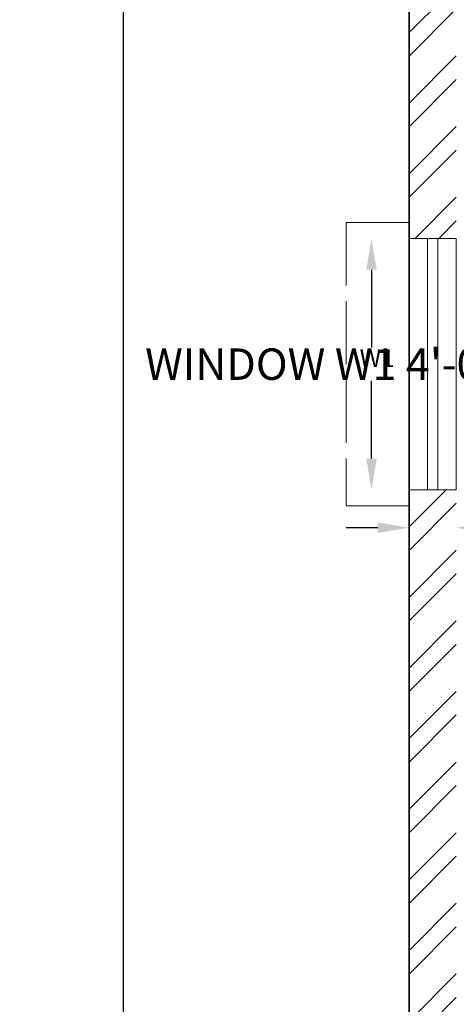
# Model space of a CAD drawing. Units: inches. Extents: x 3614 to 4242, y 2406 to 3033.
# Tile 2 of 10: x 3614 to 3697, y 2749 to 2936. Entities that reach past the tile are written whole.
import ezdxf

# ---------------------------------------------------------------- set-up
doc = ezdxf.new("R2010")
doc.units = ezdxf.units.IN
doc.linetypes.add('ACAD_ISO02W100', pattern=[15, 12, -3])
for name, color, linetype, lineweight in [('A-ANNO-DIMS', 2, 'Continuous', 18), ('A-ANNO-TEXT', 7, 'Continuous', 18), ('A-GLAZ', 4, 'Continuous', 18), ('A-GLAZ-OVHD', 8, 'ACAD_ISO02W100', 13), ('A-WALL', 7, 'Continuous', 35), ('A-WALL-PATT', 252, 'Continuous', 13)]:
    doc.layers.add(name, color=color, linetype=linetype, lineweight=lineweight)
doc.styles.get("Standard").update_dxf_attribs({"font": 'arial.ttf'})
doc.dimstyles.get("Standard").update_dxf_attribs({"dimtxt": 6, "dimasz": 6, "dimexe": 0.18, "dimexo": 0.0625, "dimgap": 0.09, "dimtad": 0, "dimtih": 1, "dimtoh": 1, "dimdec": 4, "dimzin": 0, "dimdsep": 46, "dimlunit": 4, "dimtxsty": 'Standard', "dimcen": 0.09, "dimse1": 1, "dimse2": 1, "dimadec": 0, "dimazin": 0, "dimtfac": 1, "dimtdec": 4, "dimtofl": 0, "dimtmove": 0, "dimatfit": 3, "dimfxl": 1, "dimtolj": 1, "dimtzin": 0, "dimarcsym": 0})

# ---------------------------------------------------------------- blocks, each defined once
blk = doc.blocks.new('*D26')
at = {"layer": 'A-ANNO-DIMS', "color": 0, "lineweight": -2, "transparency": 16777216}
for p, q in [((3633.72, 2948.34), (3633.72, 2707.46)), ((3633.72, 2452.14), (3633.72, 2693.02))]:
    blk.add_line(p, q, dxfattribs=at)
at = {"layer": 'A-ANNO-DIMS', "color": 0, "transparency": 16777216}
for points in [[(3632.72, 2948.34), (3634.72, 2948.34), (3633.72, 2954.34)], [(3632.72, 2452.14), (3634.72, 2452.14), (3633.72, 2446.14)]]:
    blk.add_solid(points, dxfattribs=at)
at = {"layer": 'Defpoints', "color": 0, "transparency": 16777216}
for p in [(3688.34, 2954.34), (3633.72, 2446.14), (3688.34, 2446.14)]:
    blk.add_point(p, dxfattribs=at)
at = {"layer": 'A-ANNO-DIMS', "color": 0, "transparency": 16777216, "insert": (3633.72, 2700.24), "char_height": 6, "attachment_point": 5}
blk.add_mtext('\\A1;42\'-4{\\H1x;\\S3/16;}"', dxfattribs=at)
blk = doc.blocks.new('WINDOW-W1-48IN')
for p, q in [((48, 9), (0, 9)), ((0, 9), (0, 0)), ((48, 0), (48, 9)), ((0, 5.5), (48, 5.5)), ((0, 3.5), (48, 3.5)), ((0, 0), (48, 0))]:
    blk.add_line(p, q)
blk = doc.blocks.new('SHADE-W1')
for p, q in [((0, 0), (0, 12)), ((0, 12), (51, 12)), ((51, 12), (54, 12)), ((54, 12), (54, 0)), ((3, 0), (0, 0))]:
    blk.add_line(p, q)
blk = doc.blocks.new('*D41')
at = {"layer": 'A-ANNO-DIMS', "color": 0, "lineweight": -2, "transparency": 16777216}
for p, q in [((3681.14, 2888.73), (3681.14, 2873.93)), ((3681.14, 2852.73), (3681.14, 2867.54))]:
    blk.add_line(p, q, dxfattribs=at)
at = {"layer": 'A-ANNO-DIMS', "color": 0, "transparency": 16777216}
for points in [[(3680.14, 2888.73), (3682.14, 2888.73), (3681.14, 2894.73)], [(3680.14, 2852.73), (3682.14, 2852.73), (3681.14, 2846.73)]]:
    blk.add_solid(points, dxfattribs=at)
at = {"layer": 'Defpoints', "color": 0, "transparency": 16777216}
for p in [(3688.34, 2894.73), (3681.14, 2846.73), (3688.34, 2846.73)]:
    blk.add_point(p, dxfattribs=at)
at = {"layer": 'A-ANNO-DIMS', "color": 0, "transparency": 16777216, "insert": (3681.14, 2870.73), "char_height": 6, "attachment_point": 5}
blk.add_mtext('\\A1;WINDOW W1 4\'-0" TYP.', dxfattribs=at)
blk = doc.blocks.new('*D42')
at = {"layer": 'A-ANNO-DIMS', "color": 0, "lineweight": -2, "transparency": 16777216}
for p, q in [((3682.34, 2839.53), (3676.34, 2839.53)), ((3703.34, 2839.53), (3709.34, 2839.53))]:
    blk.add_line(p, q, dxfattribs=at)
at = {"layer": 'A-ANNO-DIMS', "color": 0, "transparency": 16777216}
for points in [[(3682.34, 2840.53), (3682.34, 2838.53), (3688.34, 2839.53)], [(3703.34, 2840.53), (3703.34, 2838.53), (3697.34, 2839.53)]]:
    blk.add_solid(points, dxfattribs=at)
at = {"layer": 'Defpoints', "color": 0, "transparency": 16777216}
for p in [(3688.34, 2846.73), (3697.34, 2846.73), (3697.34, 2839.53)]:
    blk.add_point(p, dxfattribs=at)
at = {"layer": 'A-ANNO-DIMS', "color": 0, "transparency": 16777216, "insert": (3727.71, 2839.53), "char_height": 6, "attachment_point": 5}
blk.add_mtext('\\A1;0\'-9" TYP.', dxfattribs=at)

msp = doc.modelspace()

# ---------------------------------------------------------------- hatches: boundary and pattern name
at = {"layer": 'A-WALL-PATT'}
h = msp.add_hatch(dxfattribs=at)
h.set_pattern_fill('ANSI32', color=256)
h.paths.add_polyline_path([(4041.01458, 2954.34049), (3982.96188, 2954.34049), (3982.96188, 2945.34049), (3983.336, 2945.34049), (4041.01458, 2945.34049)])
h.paths.add_polyline_path([(3973.96188, 2954.34049), (3960.11861, 2954.34049), (3960.11861, 2945.34049), (3973.96188, 2945.34049)])
h.paths.add_polyline_path([(3936.11861, 2954.34049), (3901.17016, 2954.34049), (3901.17016, 2945.34049), (3913.336, 2945.34049), (3913.336, 2896.34049, -0.050382044), (3919.336, 2895.73437), (3919.336, 2945.34049), (3936.11861, 2945.34049)])
h.paths.add_polyline_path([(3983.336, 2945.34049), (3982.96188, 2945.34049), (3974.336, 2945.34049), (3974.336, 2873.34049), (3974.336, 2795.31105), (3983.336, 2795.31105), (3983.336, 2867.34049)])
h.paths.add_polyline_path([(3974.336, 2872.34049), (3919.336, 2872.34049), (3858.336, 2872.34049), (3858.336, 2866.34049), (3919.336, 2866.34049), (3974.336, 2866.34049)])
h.paths.add_polyline_path([(3877.17016, 2954.34049), (3852.34021, 2954.34049), (3852.34021, 2945.34049), (3852.336, 2896.34049), (3858.336, 2896.34049), (3858.336, 2945.34049), (3877.17016, 2945.34049)])
h.paths.add_polyline_path([(3871.94212, 2902.34049), (3858.336, 2902.34049), (3858.336, 2896.34049), (3871.336, 2896.34049, -0.050382044)], flags=0)
h.paths.add_polyline_path([(3913.336, 2902.34049), (3901.336, 2902.34049), (3901.336, 2896.34049), (3913.336, 2896.34049)], flags=17)
h.paths.add_polyline_path([(3858.336, 2872.34049), (3852.336, 2872.34049), (3852.336, 2866.34049), (3858.336, 2866.34049)])
h.paths.add_polyline_path([(3809.336, 2954.34049), (3764.4617, 2954.34049), (3764.4617, 2945.34049), (3809.336, 2945.34049)])
h.paths.add_polyline_path([(3716.4617, 2954.34049), (3697.336, 2954.34049), (3697.336, 2945.34049), (3716.4617, 2945.34049)])
h.paths.add_polyline_path([(3697.336, 2945.34049), (3688.336, 2945.34049), (3688.336, 2894.73438), (3697.336, 2894.73438)])
h = msp.add_hatch(dxfattribs=at)
h.set_pattern_fill('ANSI32', color=256)
h.paths.add_polyline_path([(4153.336, 2945.34049), (4144.336, 2945.34049), (4144.336, 2902.95478), (4153.336, 2902.95478)])
h.paths.add_polyline_path([(4144.36882, 2954.34049), (4089.01458, 2954.34049), (4089.01458, 2945.34049), (4144.36882, 2945.34049)])
h.paths.add_polyline_path([(3818.336, 2945.34049), (3809.336, 2945.34049), (3809.336, 2787.28572), (3818.336, 2787.28572)])
h.paths.add_polyline_path([(3697.336, 2846.73438), (3688.336, 2846.73438), (3688.336, 2742.34049), (3697.336, 2742.34049)])
h.paths.add_polyline_path([(3854.336, 2742.34049), (3853.36389, 2742.34049), (3818.336, 2742.34049), (3809.336, 2742.34049), (3697.336, 2742.34049), (3697.336, 2733.34049), (3809.336, 2733.34049), (3854.336, 2733.34049)])
h.paths.add_polyline_path([(3697.336, 2733.34049), (3688.336, 2733.34049), (3688.336, 2690.05693), (3697.336, 2690.05693)])
h.paths.add_polyline_path([(3697.336, 2642.05693), (3688.336, 2642.05693), (3688.336, 2583.37355), (3697.336, 2583.37355)])
h.paths.add_polyline_path([(3726.39802, 2583.34049), (3697.336, 2583.34049), (3697.336, 2574.34049), (3726.39802, 2574.34049)])
h.paths.add_polyline_path([(3842.336, 2583.34049), (3818.336, 2583.34049), (3809.336, 2583.34049), (3774.39802, 2583.34049), (3774.39802, 2574.34049), (3809.336, 2574.34049), (3842.336, 2574.34049)])
h.paths.add_polyline_path([(3890.336, 2583.34049), (3878.336, 2583.34049), (3878.336, 2574.34049), (3890.336, 2574.34049)])

# ---------------------------------------------------------------- linework, layer by layer
at = {"layer": 'A-WALL'}
msp.add_line((3688.336, 2954.34049), (3688.336, 2574.34049), dxfattribs=at)

# ---------------------------------------------------------------- block references
at = {"layer": 'A-GLAZ', "rotation": 270.000000000001}
msp.add_blockref('WINDOW-W1-48IN', (3688.33551, 2894.73408), dxfattribs=at)
at = {"layer": 'A-GLAZ-OVHD', "extrusion": (0, 0, -1), "zscale": -1, "rotation": 269.999999999997}
msp.add_blockref('SHADE-W1', (-3688.33649, 2897.73408), dxfattribs=at)

# ---------------------------------------------------------------- texts
at = {"layer": 'A-ANNO-TEXT', "insert": (3678.8741, 2873.58839), "char_height": 3.42604, "attachment_point": 1}
msp.add_mtext_dynamic_manual_height_columns('W1', width=192.8287007, gutter_width=17.1302, heights=[0], dxfattribs=at)

# ---------------------------------------------------------------- dimensions: what is measured, and where the dimension line sits
at = {"layer": 'A-ANNO-DIMS'}
dim = msp.add_linear_dim(base=(3633.71834, 2446.14049), p1=(3688.336, 2954.34049), p2=(3688.336, 2446.14049), angle=90, dimstyle='Standard', override={"dimclrd": 0, "dimclre": 0, "dimclrt": 0}, dxfattribs=at)
dim.commit()
dim.dimension.update_dxf_attribs({"geometry": '*D26', "text_midpoint": (3633.71834, 2700.24049)})
dim = msp.add_linear_dim(base=(3681.136, 2846.73438), p1=(3688.336, 2894.73438), p2=(3688.336, 2846.73438), angle=270, text='WINDOW W1 <> TYP.', dimstyle='Standard', override={"dimdec": 1, "dimlfac": 1, "dimrnd": 0, "dimzin": 1, "dimdsep": 46, "dimlunit": 4, "dimfrac": 2}, dxfattribs=at)
dim.commit()
dim.dimension.update_dxf_attribs({"geometry": '*D41', "text_midpoint": (3681.136, 2870.73438)})
dim = msp.add_linear_dim(base=(3697.336, 2839.53438), p1=(3688.336, 2846.73438), p2=(3697.336, 2846.73438), text='<> TYP.', dimstyle='Standard', override={"dimdec": 1, "dimlfac": 1, "dimrnd": 0, "dimzin": 1, "dimdsep": 46, "dimlunit": 4, "dimfrac": 2}, dxfattribs=at)
dim.commit()
dim.dimension.update_dxf_attribs({"geometry": '*D42', "text_midpoint": (3727.71249, 2839.53438)})

doc.saveas('drawing.dxf')
